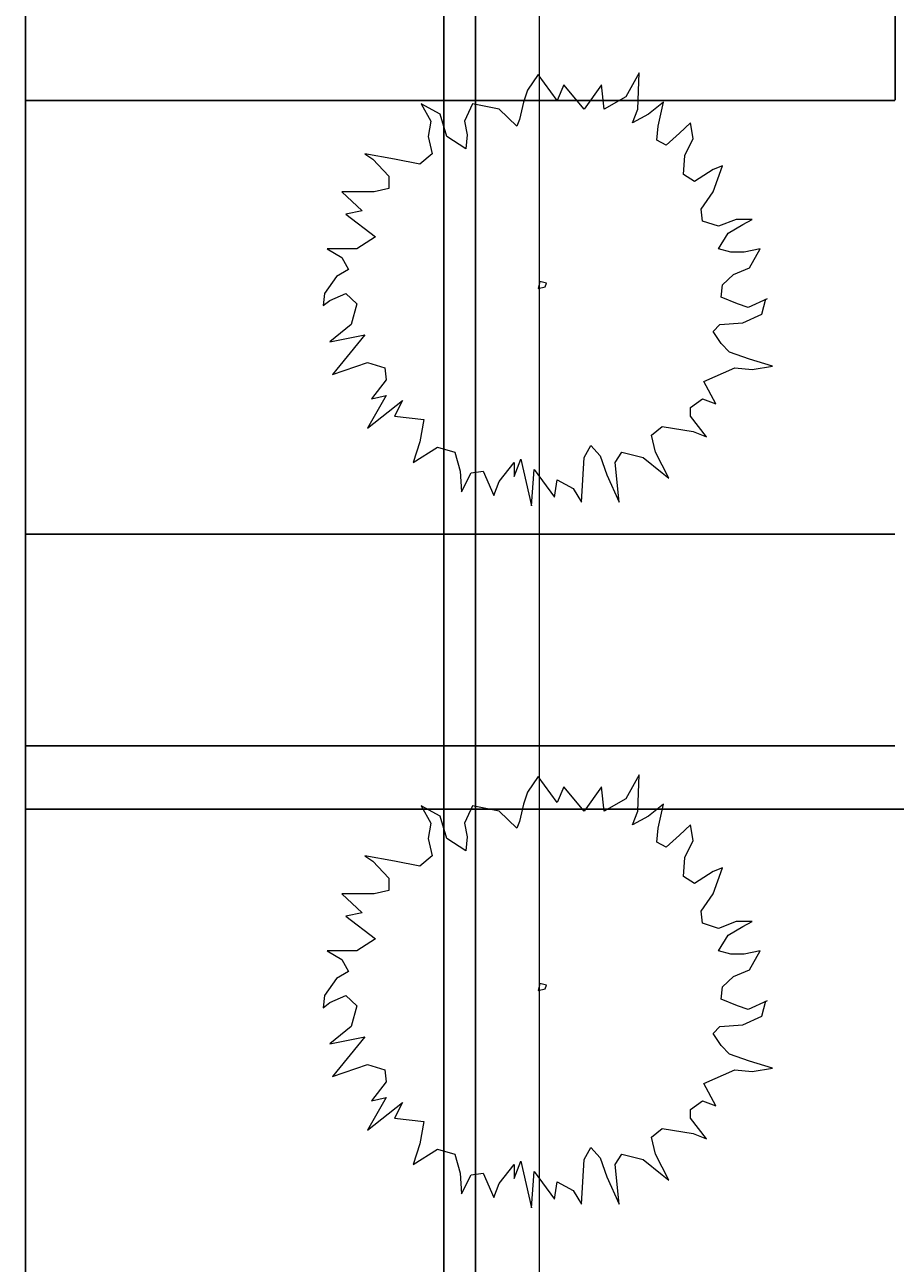
# Model space of a CAD drawing. Units: inches. Extents: x -4843 to -3402, y -164 to 3629.
# Tile 7 of 22: x -4843 to -4596, y 691 to 1042. Entities that reach past the tile are written whole.
import ezdxf

# ---------------------------------------------------------------- set-up
doc = ezdxf.new("R2010")
doc.units = ezdxf.units.IN
for name, color, linetype, lineweight in [('A-ANNO-DIMS', 2, 'Continuous', 18), ('C-PROP', 7, 'Continuous', 25), ('L-PLNT-EDGE', 7, 'Continuous', 18), ('PLANTS', 3, 'Continuous', 13)]:
    doc.layers.add(name, color=color, linetype=linetype, lineweight=lineweight)
doc.styles.get("Standard").update_dxf_attribs({"font": 'arial.ttf'})
doc.dimstyles.get("Standard").update_dxf_attribs({"dimtxt": 0.18, "dimasz": 0.18, "dimexe": 0.18, "dimexo": 0.0625, "dimgap": 0.09, "dimtad": 0, "dimtih": 1, "dimtoh": 1, "dimdec": 4, "dimzin": 0, "dimdsep": 46, "dimtxsty": 'Standard', "dimcen": 0.09, "dimadec": 0, "dimazin": 0, "dimtfac": 1, "dimtdec": 4, "dimtofl": 0, "dimtmove": 0, "dimatfit": 3, "dimfxl": 1, "dimtolj": 1, "dimtzin": 0, "dimarcsym": 0})

# ---------------------------------------------------------------- blocks, each defined once
blk = doc.blocks.new('*U34')
for points in [[(0, 1540.256), (-77.4954, 1428.4452), (-106.5784, 1341.501), (-135.636, 1217.295), (-155.0162, 1167.6126), (-280.9748, 1291.8186), (-474.7514, 1329.0804), (-532.892, 1204.8744), (-513.5118, 1105.5096), (-523.1892, 1006.1194), (-658.8506, 1093.089), (-707.2884, 1254.5568), (-842.9244, 1329.0804), (-775.1064, 1204.8744), (-794.4866, 1093.089), (-765.429, 968.8576), (-852.6272, 894.334), (-1036.701, 931.5958), (-1249.8832, 968.8576), (-1191.7426, 931.5958), (-1075.4614, 807.3898), (-1075.4614, 720.4456), (-1182.0398, 695.6044), (-1414.5768, 695.6044), (-1269.238, 558.9524), (-1385.5192, 534.1112), (-1172.3624, 372.6434), (-1307.9984, 285.6992), (-1521.1552, 285.6992), (-1414.5768, 223.5962), (-1366.139, 136.652), (-1453.3372, 86.9442), (-1540.5354, -37.2618), (-1550.2382, -124.206), (-1501.775, -86.9442), (-1385.5192, -37.2618), (-1307.9984, -111.7854), (-1346.7588, -260.8326), (-1501.775, -385.064), (-1249.8832, -335.3816), (-1482.3948, -621.0554), (-1230.503, -534.1112), (-1104.5444, -571.373), (-1094.8416, -658.3172), (-1201.42, -794.9692), (-1094.8416, -770.128), (-1230.503, -1006.1194), (-978.5858, -807.3898), (-1036.701, -919.1752), (-823.5442, -944.0164), (-852.6272, -1105.4842), (-901.065, -1254.5568), (-726.6686, -1142.746), (-600.71, -1180.0078), (-561.9496, -1316.6598), (-552.2722, -1465.707), (-484.4542, -1329.0804), (-397.2306, -1316.6598), (-319.7352, -1490.5482), (-280.9748, -1391.1834), (-174.3964, -1254.5568), (-174.3964, -1353.9216), (-125.9586, -1229.7156), (-48.4378, -1565.0718), (-29.0576, -1304.2392), (116.2812, -1502.9688), (135.6614, -1378.7628), (251.9172, -1440.8658), (310.0578, -1540.2306), (329.438, -1217.295), (377.8758, -1130.3254), (445.6938, -1204.8744), (494.157, -1341.501), (581.3552, -1540.2306), (552.2722, -1254.5568), (600.71, -1180.0078), (755.7516, -1217.295), (891.3876, -1329.0804), (939.8254, -1366.3422), (842.9498, -1180.0078), (813.8668, -1055.8018), (891.3876, -993.6988), (1114.2472, -1030.9606), (1211.1228, -1068.2224), (1094.867, -919.1752), (1094.867, -857.0722), (1182.0652, -794.9692), (1278.9408, -832.231), (1191.7426, -670.7378), (1414.6022, -571.373), (1540.5608, -583.7936), (1685.8996, -558.9524), (1521.1806, -509.27), (1375.8418, -459.5876), (1317.7012, -397.4846), (1259.5606, -310.515), (1308.0238, -260.8326), (1472.7174, -248.412), (1608.3788, -186.309), (1637.4364, -74.5236)], [(1647.1392, -74.5236), (1511.4778, -136.6266), (1433.9824, -111.7854), (1317.7012, -62.103), (1327.404, 24.8412), (1404.8994, 99.3648), (1521.1806, 149.0726), (1598.676, 285.6992), (1482.4202, 260.858), (1385.5192, 260.858), (1298.321, 285.6992), (1366.139, 397.4846), (1472.7174, 459.5876), (1540.5608, 496.8494), (1424.2796, 496.8494), (1298.321, 447.167), (1182.0652, 484.4288), (1172.3624, 571.3984), (1259.5606, 695.6044), (1327.404, 881.9134), (1259.5606, 857.0722), (1123.9246, 770.128), (1046.4038, 819.8104), (1056.1066, 956.437), (1114.2472, 1080.6684), (1094.867, 1192.4538), (1017.3462, 1117.9302), (920.4452, 1030.9606), (852.6272, 1068.2478), (862.33, 1167.6126), (901.0904, 1341.501), (794.512, 1254.5568), (678.2308, 1192.4538), (716.9912, 1291.8186), (726.6686, 1552.6766), (629.793, 1378.7628), (474.7768, 1291.8186), (455.3966, 1465.7324), (329.438, 1291.8186), (184.0992, 1465.7324), (135.6614, 1353.9216), (0, 1540.256)]]:
    blk.add_lwpolyline(points)
blk.add_lwpolyline([(9.7028, 49.6824), (0, 0), (48.4378, 12.4206), (58.1406, 37.2618)], close=True)
blk = doc.blocks.new('*D64')
at = {"layer": 'A-ANNO-DIMS', "color": 0, "lineweight": -2, "transparency": 16777216}
for p, q in [((-4595.85, 1020.35), (-4842.55, 1020.35)), ((-4842.37, 1020.17), (-4842.37, 648.04)), ((-4842.37, 275.53), (-4842.37, 647.67)), ((-4595.85, 275.35), (-4842.55, 275.35))]:
    blk.add_line(p, q, dxfattribs=at)
at = {"layer": 'A-ANNO-DIMS', "color": 0, "transparency": 16777216}
for points in [[(-4842.4, 1020.17), (-4842.34, 1020.17), (-4842.37, 1020.35)], [(-4842.4, 275.53), (-4842.34, 275.53), (-4842.37, 275.35)]]:
    blk.add_solid(points, dxfattribs=at)
at = {"layer": 'Defpoints', "color": 0, "transparency": 16777216}
for p in [(-4595.78, 1020.35), (-4842.37, 275.35), (-4595.78, 275.35)]:
    blk.add_point(p, dxfattribs=at)
at = {"layer": 'A-ANNO-DIMS', "color": 0, "transparency": 16777216, "insert": (-4842.37, 647.85), "char_height": 0.18, "attachment_point": 5}
blk.add_mtext('\\A1;745', dxfattribs=at)
blk = doc.blocks.new('*D68')
at = {"layer": 'A-ANNO-DIMS', "color": 0, "lineweight": -2, "transparency": 16777216}
for p, q in [((-4723.85, 1149.35), (-4842.55, 1149.35)), ((-4842.37, 1149.17), (-4842.37, 1085.04)), ((-4842.37, 1020.53), (-4842.37, 1084.67)), ((-4595.85, 1020.35), (-4842.55, 1020.35))]:
    blk.add_line(p, q, dxfattribs=at)
at = {"layer": 'A-ANNO-DIMS', "color": 0, "transparency": 16777216}
for points in [[(-4842.4, 1149.17), (-4842.34, 1149.17), (-4842.37, 1149.35)], [(-4842.4, 1020.53), (-4842.34, 1020.53), (-4842.37, 1020.35)]]:
    blk.add_solid(points, dxfattribs=at)
at = {"layer": 'Defpoints', "color": 0, "transparency": 16777216}
for p in [(-4723.78, 1149.35), (-4842.37, 1020.35), (-4595.78, 1020.35)]:
    blk.add_point(p, dxfattribs=at)
at = {"layer": 'A-ANNO-DIMS', "color": 0, "transparency": 16777216, "insert": (-4842.37, 1084.85), "char_height": 0.18, "attachment_point": 5}
blk.add_mtext('\\A1;129', dxfattribs=at)
blk = doc.blocks.new('*D69')
at = {"layer": 'A-ANNO-DIMS', "color": 0, "lineweight": -2, "transparency": 16777216}
for p, q in [((-4595.78, 1020.42), (-4595.78, 1392.95)), ((-4595.6, 1392.77), (-4537.56, 1392.77)), ((-4478.96, 1392.77), (-4537, 1392.77)), ((-4478.78, 1020.42), (-4478.78, 1392.95))]:
    blk.add_line(p, q, dxfattribs=at)
at = {"layer": 'A-ANNO-DIMS', "color": 0, "transparency": 16777216}
for points in [[(-4595.6, 1392.8), (-4595.6, 1392.74), (-4595.78, 1392.77)], [(-4478.96, 1392.8), (-4478.96, 1392.74), (-4478.78, 1392.77)]]:
    blk.add_solid(points, dxfattribs=at)
at = {"layer": 'Defpoints', "color": 0, "transparency": 16777216}
for p in [(-4478.78, 1392.77), (-4595.78, 1020.35), (-4478.78, 1020.35)]:
    blk.add_point(p, dxfattribs=at)
at = {"layer": 'A-ANNO-DIMS', "color": 0, "transparency": 16777216, "insert": (-4537.28, 1392.77), "char_height": 0.18, "attachment_point": 5}
blk.add_mtext('\\A1;117', dxfattribs=at)
blk = doc.blocks.new('*D73')
at = {"layer": 'A-ANNO-DIMS', "color": 0, "lineweight": -2, "transparency": 16777216}
for p, q in [((-4595.85, 1020.35), (-4842.55, 1020.35)), ((-4842.37, 1020.17), (-4842.37, 959.04)), ((-4842.37, 897.53), (-4842.37, 958.67)), ((-4595.85, 897.35), (-4842.55, 897.35))]:
    blk.add_line(p, q, dxfattribs=at)
at = {"layer": 'A-ANNO-DIMS', "color": 0, "transparency": 16777216}
for points in [[(-4842.4, 1020.17), (-4842.34, 1020.17), (-4842.37, 1020.35)], [(-4842.4, 897.53), (-4842.34, 897.53), (-4842.37, 897.35)]]:
    blk.add_solid(points, dxfattribs=at)
at = {"layer": 'Defpoints', "color": 0, "transparency": 16777216}
for p in [(-4595.78, 1020.35), (-4842.37, 897.35), (-4595.78, 897.35)]:
    blk.add_point(p, dxfattribs=at)
at = {"layer": 'A-ANNO-DIMS', "color": 0, "transparency": 16777216, "insert": (-4842.37, 958.85), "char_height": 0.18, "attachment_point": 5}
blk.add_mtext('\\A1;123', dxfattribs=at)
blk = doc.blocks.new('*D74')
at = {"layer": 'A-ANNO-DIMS', "color": 0, "lineweight": -2, "transparency": 16777216}
for p, q in [((-4595.85, 837.35), (-4842.55, 837.35)), ((-4842.37, 837.17), (-4842.37, 828.54)), ((-4842.37, 819.53), (-4842.37, 828.17)), ((-4586.85, 819.35), (-4842.55, 819.35))]:
    blk.add_line(p, q, dxfattribs=at)
at = {"layer": 'A-ANNO-DIMS', "color": 0, "transparency": 16777216}
for points in [[(-4842.4, 837.17), (-4842.34, 837.17), (-4842.37, 837.35)], [(-4842.4, 819.53), (-4842.34, 819.53), (-4842.37, 819.35)]]:
    blk.add_solid(points, dxfattribs=at)
at = {"layer": 'Defpoints', "color": 0, "transparency": 16777216}
for p in [(-4595.78, 837.35), (-4842.37, 819.35), (-4586.78, 819.35)]:
    blk.add_point(p, dxfattribs=at)
at = {"layer": 'A-ANNO-DIMS', "color": 0, "transparency": 16777216, "insert": (-4842.37, 828.35), "char_height": 0.18, "attachment_point": 5}
blk.add_mtext('\\A1;18', dxfattribs=at)

msp = doc.modelspace()

# ---------------------------------------------------------------- linework, layer by layer
at = {"layer": 'C-PROP'}
for p, q in [((-4723.78, 1149.35), (-4723.78, 86.35)), ((-4714.78, 1140.35), (-4714.78, 95.35))]:
    msp.add_line(p, q, dxfattribs=at)
at = {"layer": 'L-PLNT-EDGE'}
msp.add_line((-4696.78, 1116.35), (-4696.78, 95.35), dxfattribs=at)

# ---------------------------------------------------------------- block references
at = {"layer": 'PLANTS', "xscale": 0.0393700787401575, "yscale": 0.0393700787401575, "zscale": 0.0393700787401575}
for p in [(-4696.97, 967.02), (-4696.97, 767.96)]:
    msp.add_blockref('*U34', p, dxfattribs=at)

# ---------------------------------------------------------------- dimensions: what is measured, and where the dimension line sits
at = {"layer": 'A-ANNO-DIMS'}
dim = msp.add_linear_dim(base=(-4478.78, 1392.77), p1=(-4595.78, 1020.35), p2=(-4478.78, 1020.35), dimstyle='Standard', override={"dimdec": 0, "dimlfac": 1, "dimrnd": 0, "dimzin": 0, "dimdsep": 46, "dimlunit": 2}, dxfattribs=at)
dim.commit()
dim.dimension.update_dxf_attribs({"geometry": '*D69', "text_midpoint": (-4537.28, 1392.77)})
for base, p1, p2, picture, middle in [((-4842.37, 1020.35), (-4723.78, 1149.35), (-4595.78, 1020.35), '*D68', (-4842.37, 1084.85)), ((-4842.37, 275.35), (-4595.78, 1020.35), (-4595.78, 275.35), '*D64', (-4842.37, 647.85)), ((-4842.37, 897.35), (-4595.78, 1020.35), (-4595.78, 897.35), '*D73', (-4842.37, 958.85)), ((-4842.37, 819.35), (-4595.78, 837.35), (-4586.78, 819.35), '*D74', (-4842.37, 828.35))]:
    dim = msp.add_linear_dim(base=base, p1=p1, p2=p2, angle=90, dimstyle='Standard', override={"dimdec": 0, "dimlfac": 1, "dimrnd": 0, "dimzin": 0, "dimdsep": 46, "dimlunit": 2}, dxfattribs=at)
    dim.commit()
    dim.dimension.update_dxf_attribs({"geometry": picture, "text_midpoint": middle})

doc.saveas('drawing.dxf')
